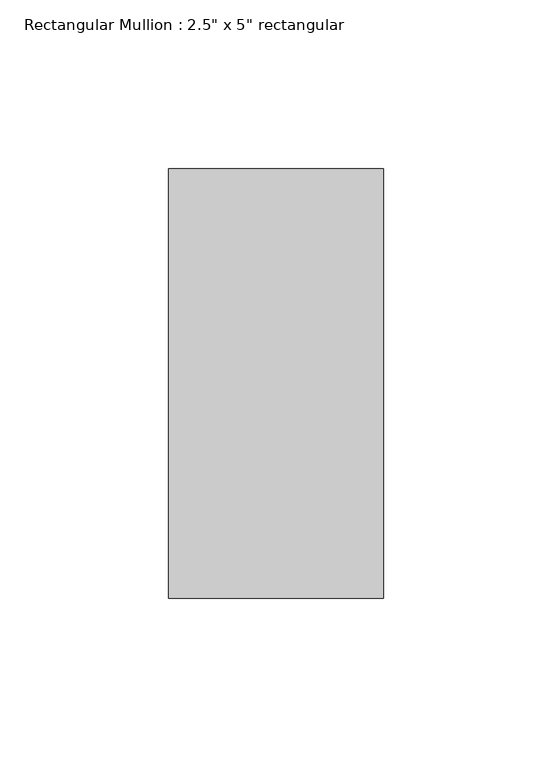
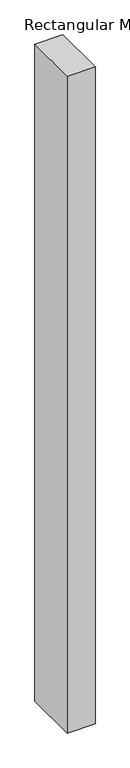
"""IFC4 building model written with IfcOpenShell, lengths in millimetres: member geometry."""

from ifc_helpers import new_model, si_unit, frame, origin, place, context, project, spatial, polyline, outline, extrude, source, transform, mapped, element, save


def member_d6231c0b(model_context):
    return source(origin(), model_context, "Body", "SweptSolid", [
        extrude(outline(polyline([(0.0, 63.5), (0.0, -63.5), (-63.5, -63.5), (-63.5, 63.5), (0.0, 63.5)])), frame((0.0, 0.0, -1579.7129991), z_axis=(0.0, 0.0, 1.0), x_axis=(1.0, 0.0, 0.0)), (0.0, 0.0, 1.0), 1579.7129991),
    ])


if __name__ == "__main__":
    model = new_model("IFC4")
    model_context = context("Model", 3, world=origin())
    ifc_project = project(units=[si_unit("LENGTHUNIT", "METRE", prefix="MILLI")], contexts=[model_context])
    site = spatial("IfcSite", under=ifc_project)
    building = spatial("IfcBuilding", under=site)
    placement = place(None, origin())
    member_shape = member_d6231c0b(model_context)
    element("IfcMember", 1, ObjectType="Rectangular Mullion : 2.5\" x 5\" rectangular", at=placement, inside=building, context=model_context, shape_type="MappedRepresentation", body=[
        mapped(member_shape, transform((0.0, 0.0, 0.0), x_axis=(1.0, 0.0, 0.0), y_axis=(0.0, 1.0, 0.0), z_axis=(0.0, 0.0, 1.0))),
    ])
    save(model, "model.ifc")

# Revit data of these elements
# Type "Rectangular Mullion : 2.5\" x 5\" rectangular"
#   built-in parameter 1007304 = 0.416667 (stored number, unit not read)
#   built-in parameter 1007301 = 0.104167 (stored number, unit not read)
#   built-in parameter 1007300 = 0.104167 (stored number, unit not read)
# Element 1 (IfcMember, "Rectangular Mullion : 2.5\" x 5\" rectangular")
#   Materials on its faces: "Aluminum"
# Materials
#   "Aluminum": class "Metal", colour RGB 247 247 247, transparency 0, Description = "Aluminum 6061", Cost = 0
